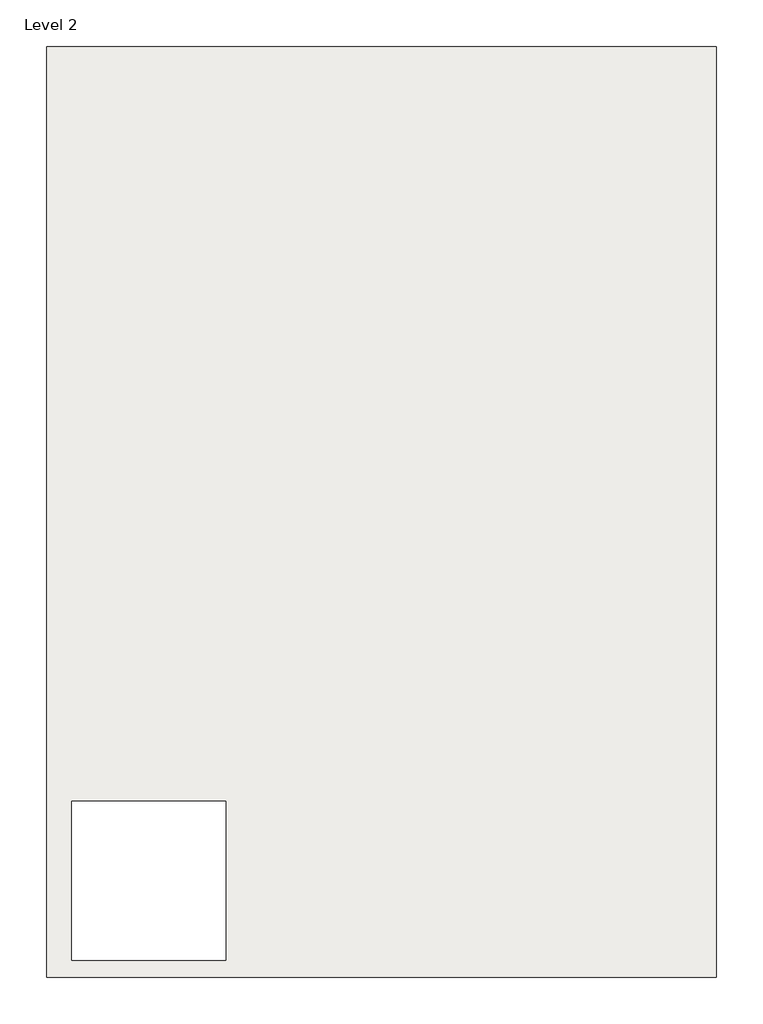
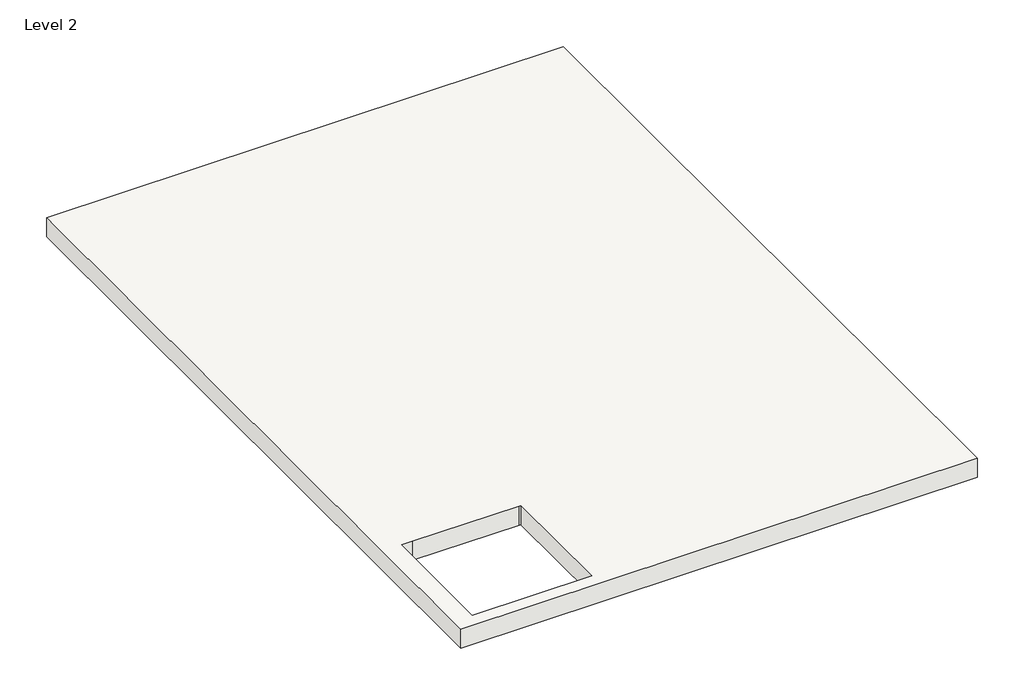
# One storey: 1 roof.
"""IFC4 building model written with IfcOpenShell, lengths in millimetres."""

from ifc_helpers import new_model, si_unit, frame, origin, place, context, project, spatial, polyline, outline, extrude, element, save

model = new_model("IFC4")

# Units and contexts
model_context = context("Model", 3, world=origin())
ifc_project = project(units=[si_unit("LENGTHUNIT", "METRE", prefix="MILLI")], contexts=[model_context])

# Site, building, storey
site = spatial("IfcSite", under=ifc_project)
building = spatial("IfcBuilding", under=site)
storey = spatial("IfcBuildingStorey", under=building, Name="Level 2", Elevation=3048.0)

# Roof
placement = place(None, origin())
element("IfcRoof", 1, ObjectType="Generic - 12\"", at=placement, inside=storey, context=model_context, shape_type="SweptSolid", body=[
    extrude(outline(polyline([(-13057.0047602, 14148.499435), (-5233.8047602, 14148.499435), (-5233.8047602, 3277.299435), (-13057.0047602, 3277.299435), (-13057.0047602, 14148.499435)]), holes=[polyline([(-10961.5047602, 5334.699435), (-10986.9047602, 5334.699435), (-12603.5364521, 5334.699435), (-12764.9047602, 5334.699435), (-12764.9047602, 3480.499435), (-10961.5047602, 3480.499435), (-10961.5047602, 5334.699435)])]), frame((0.0, 0.0, 3048.0), z_axis=(0.0, 0.0, 1.0), x_axis=(1.0, 0.0, 0.0)), (0.0, 0.0, 1.0), 304.8),
])

save(model, "model.ifc")

# Revit data of these elements
# Type "Generic - 12\""
#   Assembly Code = "B1020"
#   Layers, outside or top first: 1' - 0" "Brick, Soldier Course" (function 1)
# Element 1 (IfcRoof, "Generic - 12\"")
#   built-in parameter 1001705 = 11 (stored number, unit not read)
#   built-in parameter 1001710 = 33615
#   Phase Created = New Construction
#   Materials on its faces: "Brick, Soldier Course"
# Materials
#   "Brick, Soldier Course": class "Masonry", colour RGB 170 98 104, transparency 0, Description = "Common brick soldier coursed", Cost = 0
